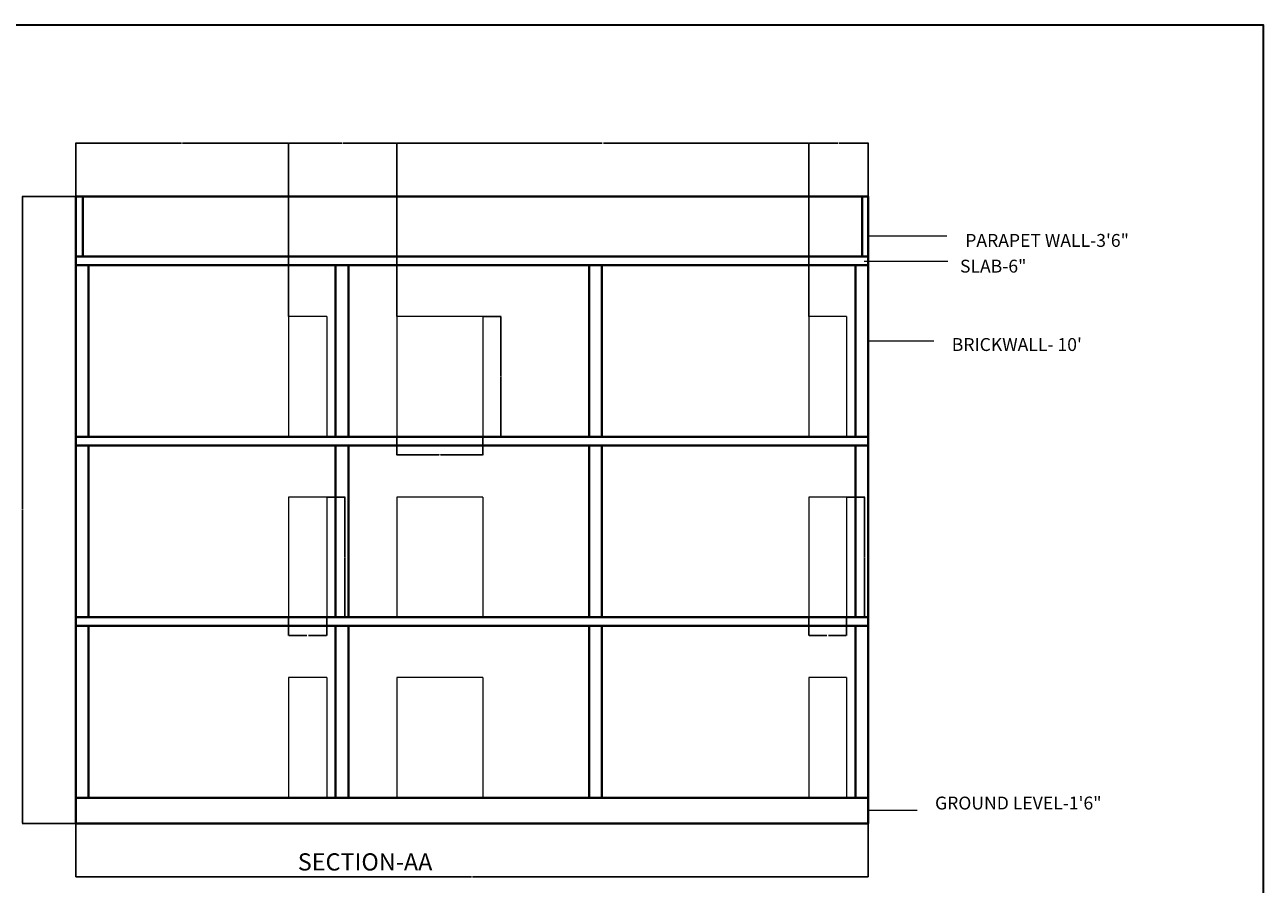
# Model space of a CAD drawing. Units: inches. Extents: x 2014 to 3678, y 870 to 2323.
# Tile 7 of 7: x 2813 to 3678, y 1723 to 2323. Entities that reach past the tile are written whole.
import ezdxf

# ---------------------------------------------------------------- set-up
doc = ezdxf.new("R2010")
doc.units = ezdxf.units.IN
for name, color, linetype, lineweight in [('A-ANNO-DIMS', 2, 'Continuous', 18), ('A-ANNO-SYMB', 2, 'Continuous', 18), ('A-ANNO-TEXT', 7, 'Continuous', 18), ('A-ANNO-TTLB', 7, 'Continuous', 35), ('A-SECT', 7, 'Continuous', 40), ('A-SECT-OPEN', 4, 'Continuous', 18)]:
    doc.layers.add(name, color=color, linetype=linetype, lineweight=lineweight)
doc.styles.get("Standard").update_dxf_attribs({"font": 'arial.ttf'})
doc.dimstyles.get("Standard").update_dxf_attribs({"dimtxt": 0.18, "dimasz": 0.18, "dimexe": 0.18, "dimexo": 0.0625, "dimgap": 0.09, "dimtad": 0, "dimtih": 1, "dimtoh": 1, "dimdec": 4, "dimzin": 0, "dimdsep": 46, "dimtxsty": 'Standard', "dimcen": 0.09, "dimadec": 0, "dimazin": 0, "dimtfac": 1, "dimtdec": 4, "dimtofl": 0, "dimtmove": 0, "dimatfit": 3, "dimfxl": 1, "dimtolj": 1, "dimtzin": 0, "dimarcsym": 0})

# ---------------------------------------------------------------- blocks, each defined once
blk = doc.blocks.new('SECT-OPENING-LAV-EAST')
for p, q in [((0, 84), (0, 0)), ((26.34, 84), (0, 84)), ((26.34, 84), (26.34, 0))]:
    blk.add_line(p, q)
blk = doc.blocks.new('SECT-OPENING-LAV-WEST')
for p, q in [((0, 84), (0, 0)), ((26.83, 84), (0, 84)), ((26.83, 84), (26.83, 0))]:
    blk.add_line(p, q)
blk = doc.blocks.new('SECT-OPENING-BED')
for p, q in [((0, 84), (0, 0)), ((60, 84), (0, 84)), ((60, 84), (60, 0))]:
    blk.add_line(p, q)
blk = doc.blocks.new('*D80')
at = {"layer": 'A-ANNO-DIMS', "color": 0, "lineweight": -2, "transparency": 16777216}
for p, q in [((3387.07, 1993.52), (3399.78, 1993.52)), ((3399.6, 1993.34), (3399.6, 1951.71)), ((3399.6, 1909.7), (3399.6, 1951.34)), ((3387.07, 1909.52), (3399.78, 1909.52))]:
    blk.add_line(p, q, dxfattribs=at)
at = {"layer": 'A-ANNO-DIMS', "color": 0, "transparency": 16777216}
for points in [[(3399.57, 1993.34), (3399.63, 1993.34), (3399.6, 1993.52)], [(3399.57, 1909.7), (3399.63, 1909.7), (3399.6, 1909.52)]]:
    blk.add_solid(points, dxfattribs=at)
at = {"layer": 'Defpoints', "color": 0, "transparency": 16777216}
for p in [(3387, 1993.52), (3399.6, 1993.52), (3387, 1909.52)]:
    blk.add_point(p, dxfattribs=at)
at = {"layer": 'A-ANNO-DIMS', "color": 0, "transparency": 16777216, "insert": (3399.6, 1951.52), "char_height": 0.18, "attachment_point": 5}
blk.add_mtext('\\A1;OPENING 84 TYP.', dxfattribs=at)
blk = doc.blocks.new('*D81')
at = {"layer": 'A-ANNO-DIMS', "color": 0, "lineweight": -2, "transparency": 16777216}
for p, q in [((3360.66, 1909.46), (3360.66, 1896.74)), ((3387, 1909.46), (3387, 1896.74)), ((3360.84, 1896.92), (3373.31, 1896.92)), ((3386.82, 1896.92), (3374.36, 1896.92))]:
    blk.add_line(p, q, dxfattribs=at)
at = {"layer": 'A-ANNO-DIMS', "color": 0, "transparency": 16777216}
for points in [[(3360.84, 1896.95), (3360.84, 1896.89), (3360.66, 1896.92)], [(3386.82, 1896.95), (3386.82, 1896.89), (3387, 1896.92)]]:
    blk.add_solid(points, dxfattribs=at)
at = {"layer": 'Defpoints', "color": 0, "transparency": 16777216}
for p in [(3360.66, 1909.52), (3387, 1909.52), (3387, 1896.92)]:
    blk.add_point(p, dxfattribs=at)
at = {"layer": 'A-ANNO-DIMS', "color": 0, "transparency": 16777216, "insert": (3373.83, 1896.92), "char_height": 0.18, "attachment_point": 5}
blk.add_mtext('\\A1;26 TYP.', dxfattribs=at)
blk = doc.blocks.new('*D82')
at = {"layer": 'A-ANNO-DIMS', "color": 0, "lineweight": -2, "transparency": 16777216}
for p, q in [((3024.17, 1993.52), (3036.89, 1993.52)), ((3036.71, 1993.34), (3036.71, 1951.71)), ((3036.71, 1909.7), (3036.71, 1951.34)), ((3024.17, 1909.52), (3036.89, 1909.52))]:
    blk.add_line(p, q, dxfattribs=at)
at = {"layer": 'A-ANNO-DIMS', "color": 0, "transparency": 16777216}
for points in [[(3036.68, 1993.34), (3036.74, 1993.34), (3036.71, 1993.52)], [(3036.68, 1909.7), (3036.74, 1909.7), (3036.71, 1909.52)]]:
    blk.add_solid(points, dxfattribs=at)
at = {"layer": 'Defpoints', "color": 0, "transparency": 16777216}
for p in [(3024.11, 1993.52), (3036.71, 1993.52), (3024.11, 1909.52)]:
    blk.add_point(p, dxfattribs=at)
at = {"layer": 'A-ANNO-DIMS', "color": 0, "transparency": 16777216, "insert": (3036.71, 1951.52), "char_height": 0.18, "attachment_point": 5}
blk.add_mtext('\\A1;OPENING 84 TYP.', dxfattribs=at)
blk = doc.blocks.new('*D83')
at = {"layer": 'A-ANNO-DIMS', "color": 0, "lineweight": -2, "transparency": 16777216}
for p, q in [((2997.28, 1909.46), (2997.28, 1896.74)), ((3024.11, 1909.46), (3024.11, 1896.74)), ((2997.46, 1896.92), (3010.16, 1896.92)), ((3023.93, 1896.92), (3011.22, 1896.92))]:
    blk.add_line(p, q, dxfattribs=at)
at = {"layer": 'A-ANNO-DIMS', "color": 0, "transparency": 16777216}
for points in [[(2997.46, 1896.95), (2997.46, 1896.89), (2997.28, 1896.92)], [(3023.93, 1896.95), (3023.93, 1896.89), (3024.11, 1896.92)]]:
    blk.add_solid(points, dxfattribs=at)
at = {"layer": 'Defpoints', "color": 0, "transparency": 16777216}
for p in [(2997.28, 1909.52), (3024.11, 1909.52), (3024.11, 1896.92)]:
    blk.add_point(p, dxfattribs=at)
at = {"layer": 'A-ANNO-DIMS', "color": 0, "transparency": 16777216, "insert": (3010.69, 1896.92), "char_height": 0.18, "attachment_point": 5}
blk.add_mtext('\\A1;27 TYP.', dxfattribs=at)
blk = doc.blocks.new('*D84')
at = {"layer": 'A-ANNO-DIMS', "color": 0, "lineweight": -2, "transparency": 16777216}
for p, q in [((3132.99, 2119.52), (3145.71, 2119.52)), ((3145.53, 2119.34), (3145.53, 2077.71)), ((3145.53, 2035.7), (3145.53, 2077.34)), ((3132.99, 2035.52), (3145.71, 2035.52))]:
    blk.add_line(p, q, dxfattribs=at)
at = {"layer": 'A-ANNO-DIMS', "color": 0, "transparency": 16777216}
for points in [[(3145.5, 2119.34), (3145.56, 2119.34), (3145.53, 2119.52)], [(3145.5, 2035.7), (3145.56, 2035.7), (3145.53, 2035.52)]]:
    blk.add_solid(points, dxfattribs=at)
at = {"layer": 'Defpoints', "color": 0, "transparency": 16777216}
for p in [(3132.93, 2119.52), (3145.53, 2119.52), (3132.93, 2035.52)]:
    blk.add_point(p, dxfattribs=at)
at = {"layer": 'A-ANNO-DIMS', "color": 0, "transparency": 16777216, "insert": (3145.53, 2077.52), "char_height": 0.18, "attachment_point": 5}
blk.add_mtext('\\A1;OPENING 84 TYP.', dxfattribs=at)
blk = doc.blocks.new('*D85')
at = {"layer": 'A-ANNO-DIMS', "color": 0, "lineweight": -2, "transparency": 16777216}
for p, q in [((3072.93, 2035.46), (3072.93, 2022.74)), ((3132.93, 2035.46), (3132.93, 2022.74)), ((3073.11, 2022.92), (3102.4, 2022.92)), ((3132.75, 2022.92), (3103.45, 2022.92))]:
    blk.add_line(p, q, dxfattribs=at)
at = {"layer": 'A-ANNO-DIMS', "color": 0, "transparency": 16777216}
for points in [[(3073.11, 2022.95), (3073.11, 2022.89), (3072.93, 2022.92)], [(3132.75, 2022.95), (3132.75, 2022.89), (3132.93, 2022.92)]]:
    blk.add_solid(points, dxfattribs=at)
at = {"layer": 'Defpoints', "color": 0, "transparency": 16777216}
for p in [(3072.93, 2035.52), (3132.93, 2035.52), (3132.93, 2022.92)]:
    blk.add_point(p, dxfattribs=at)
at = {"layer": 'A-ANNO-DIMS', "color": 0, "transparency": 16777216, "insert": (3102.93, 2022.92), "char_height": 0.18, "attachment_point": 5}
blk.add_mtext('\\A1;60 TYP.', dxfattribs=at)
blk = doc.blocks.new('*D114')
at = {"layer": 'A-ANNO-DIMS', "color": 0, "lineweight": -2, "transparency": 16777216}
for p, q in [((2848.67, 1765.46), (2848.67, 1728.19)), ((3402.17, 1765.46), (3402.17, 1728.19)), ((2848.85, 1728.37), (3125.03, 1728.37)), ((3401.99, 1728.37), (3125.82, 1728.37))]:
    blk.add_line(p, q, dxfattribs=at)
at = {"layer": 'A-ANNO-DIMS', "color": 0, "transparency": 16777216}
for points in [[(2848.85, 1728.4), (2848.85, 1728.34), (2848.67, 1728.37)], [(3401.99, 1728.4), (3401.99, 1728.34), (3402.17, 1728.37)]]:
    blk.add_solid(points, dxfattribs=at)
at = {"layer": 'Defpoints', "color": 0, "transparency": 16777216}
for p in [(2848.67, 1765.52), (3402.17, 1765.52), (3402.17, 1728.37)]:
    blk.add_point(p, dxfattribs=at)
at = {"layer": 'A-ANNO-DIMS', "color": 0, "transparency": 16777216, "insert": (3125.42, 1728.37), "char_height": 0.18, "attachment_point": 5}
blk.add_mtext('\\A1;553.5', dxfattribs=at)
blk = doc.blocks.new('*D115')
at = {"layer": 'A-ANNO-DIMS', "color": 0, "lineweight": -2, "transparency": 16777216}
for p, q in [((2848.61, 2203.52), (2811.34, 2203.52)), ((2811.52, 2203.34), (2811.52, 1984.71)), ((2811.52, 1765.7), (2811.52, 1984.34)), ((2848.61, 1765.52), (2811.34, 1765.52))]:
    blk.add_line(p, q, dxfattribs=at)
at = {"layer": 'A-ANNO-DIMS', "color": 0, "transparency": 16777216}
for points in [[(2811.49, 2203.34), (2811.55, 2203.34), (2811.52, 2203.52)], [(2811.49, 1765.7), (2811.55, 1765.7), (2811.52, 1765.52)]]:
    blk.add_solid(points, dxfattribs=at)
at = {"layer": 'Defpoints', "color": 0, "transparency": 16777216}
for p in [(2811.52, 2203.52), (2848.67, 2203.52), (2848.67, 1765.52)]:
    blk.add_point(p, dxfattribs=at)
at = {"layer": 'A-ANNO-DIMS', "color": 0, "transparency": 16777216, "insert": (2811.52, 1984.52), "char_height": 0.18, "attachment_point": 5}
blk.add_mtext('\\A1;438', dxfattribs=at)
blk = doc.blocks.new('*D116')
at = {"layer": 'A-ANNO-DIMS', "color": 0, "lineweight": -2, "transparency": 16777216}
for p, q in [((2848.67, 2203.59), (2848.67, 2240.85)), ((2848.85, 2240.67), (2922.59, 2240.67)), ((2997.1, 2240.67), (2923.36, 2240.67)), ((2997.28, 2119.59), (2997.28, 2240.85))]:
    blk.add_line(p, q, dxfattribs=at)
at = {"layer": 'A-ANNO-DIMS', "color": 0, "transparency": 16777216}
for points in [[(2848.85, 2240.7), (2848.85, 2240.64), (2848.67, 2240.67)], [(2997.1, 2240.7), (2997.1, 2240.64), (2997.28, 2240.67)]]:
    blk.add_solid(points, dxfattribs=at)
at = {"layer": 'Defpoints', "color": 0, "transparency": 16777216}
for p in [(2997.28, 2240.67), (2848.67, 2203.52), (2997.28, 2119.52)]:
    blk.add_point(p, dxfattribs=at)
at = {"layer": 'A-ANNO-DIMS', "color": 0, "transparency": 16777216, "insert": (2922.97, 2240.67), "char_height": 0.18, "attachment_point": 5}
blk.add_mtext('\\A1;148.6', dxfattribs=at)
blk = doc.blocks.new('*D117')
at = {"layer": 'A-ANNO-DIMS', "color": 0, "lineweight": -2, "transparency": 16777216}
for p, q in [((2997.28, 2119.59), (2997.28, 2240.85)), ((2997.46, 2240.67), (3034.71, 2240.67)), ((3072.75, 2240.67), (3035.49, 2240.67)), ((3072.93, 2119.59), (3072.93, 2240.85))]:
    blk.add_line(p, q, dxfattribs=at)
at = {"layer": 'A-ANNO-DIMS', "color": 0, "transparency": 16777216}
for points in [[(2997.46, 2240.7), (2997.46, 2240.64), (2997.28, 2240.67)], [(3072.75, 2240.7), (3072.75, 2240.64), (3072.93, 2240.67)]]:
    blk.add_solid(points, dxfattribs=at)
at = {"layer": 'Defpoints', "color": 0, "transparency": 16777216}
for p in [(3072.93, 2240.67), (2997.28, 2119.52), (3072.93, 2119.52)]:
    blk.add_point(p, dxfattribs=at)
at = {"layer": 'A-ANNO-DIMS', "color": 0, "transparency": 16777216, "insert": (3035.1, 2240.67), "char_height": 0.18, "attachment_point": 5}
blk.add_mtext('\\A1;75.65', dxfattribs=at)
blk = doc.blocks.new('*D118')
at = {"layer": 'A-ANNO-DIMS', "color": 0, "lineweight": -2, "transparency": 16777216}
for p, q in [((3072.93, 2119.59), (3072.93, 2240.85)), ((3073.11, 2240.67), (3216.33, 2240.67)), ((3360.48, 2240.67), (3217.26, 2240.67)), ((3360.66, 2119.59), (3360.66, 2240.85))]:
    blk.add_line(p, q, dxfattribs=at)
at = {"layer": 'A-ANNO-DIMS', "color": 0, "transparency": 16777216}
for points in [[(3073.11, 2240.7), (3073.11, 2240.64), (3072.93, 2240.67)], [(3360.48, 2240.7), (3360.48, 2240.64), (3360.66, 2240.67)]]:
    blk.add_solid(points, dxfattribs=at)
at = {"layer": 'Defpoints', "color": 0, "transparency": 16777216}
for p in [(3360.66, 2240.67), (3072.93, 2119.52), (3360.66, 2119.52)]:
    blk.add_point(p, dxfattribs=at)
at = {"layer": 'A-ANNO-DIMS', "color": 0, "transparency": 16777216, "insert": (3216.8, 2240.67), "char_height": 0.18, "attachment_point": 5}
blk.add_mtext('\\A1;287.74', dxfattribs=at)
blk = doc.blocks.new('*D119')
at = {"layer": 'A-ANNO-DIMS', "color": 0, "lineweight": -2, "transparency": 16777216}
for p, q in [((3360.66, 2119.59), (3360.66, 2240.85)), ((3360.84, 2240.67), (3381.04, 2240.67)), ((3401.99, 2240.67), (3381.8, 2240.67)), ((3402.17, 2203.59), (3402.17, 2240.85))]:
    blk.add_line(p, q, dxfattribs=at)
at = {"layer": 'A-ANNO-DIMS', "color": 0, "transparency": 16777216}
for points in [[(3360.84, 2240.7), (3360.84, 2240.64), (3360.66, 2240.67)], [(3401.99, 2240.7), (3401.99, 2240.64), (3402.17, 2240.67)]]:
    blk.add_solid(points, dxfattribs=at)
at = {"layer": 'Defpoints', "color": 0, "transparency": 16777216}
for p in [(3402.17, 2240.67), (3402.17, 2203.52), (3360.66, 2119.52)]:
    blk.add_point(p, dxfattribs=at)
at = {"layer": 'A-ANNO-DIMS', "color": 0, "transparency": 16777216, "insert": (3381.42, 2240.67), "char_height": 0.18, "attachment_point": 5}
blk.add_mtext('\\A1;41.51', dxfattribs=at)

msp = doc.modelspace()

# ---------------------------------------------------------------- linework, layer by layer
at = {"layer": 'A-ANNO-SYMB'}
for p, q in [((3402.1718, 2175.8362), (3456.966, 2175.8362)), ((3399.338, 2158.1977), (3457.7977, 2158.1977)), ((3402.1718, 2102.5752), (3448.0271, 2102.5752)), ((3402.1718, 1774.9062), (3436.4174, 1774.9062))]:
    msp.add_line(p, q, dxfattribs=at)
at = {"layer": 'A-ANNO-TTLB'}
msp.add_lwpolyline([(2014.0556, 2323.3638), (3678.0069, 2323.3638), (3678.0069, 869.855), (2014.0556, 869.855)], close=True, dxfattribs=at)
at = {"layer": 'A-SECT'}
for p, q in [((2848.6718, 2203.5235), (2848.6718, 2017.5235)), ((3402.1718, 2203.5235), (2848.6718, 2203.5235)), ((2853.6051, 2161.5235), (2853.6051, 2203.5235)), ((3397.8601, 2161.5235), (3397.8601, 2203.5235)), ((3402.1718, 2203.5235), (3402.1718, 2017.5235)), ((3402.1718, 2161.5235), (2848.6718, 2161.5235)), ((3402.1718, 2155.5235), (2848.6718, 2155.5235)), ((2857.6718, 2155.5235), (2857.6718, 2035.5235)), ((3030.1718, 2155.5235), (3030.1718, 2035.5235)), ((3039.1718, 2155.5235), (3039.1718, 2035.5235)), ((3207.1718, 2155.5235), (3207.1718, 2035.5235)), ((3216.1718, 2155.5235), (3216.1718, 2035.5235)), ((3393.1718, 2155.5235), (3393.1718, 2035.5235)), ((2848.6718, 2077.5235), (2848.6718, 1891.5235)), ((3402.1718, 2077.5235), (3402.1718, 1891.5235)), ((3402.1718, 2035.5235), (2848.6718, 2035.5235)), ((3402.1718, 2029.5235), (2848.6718, 2029.5235)), ((2857.6718, 2029.5235), (2857.6718, 1909.5235)), ((3030.1718, 2029.5235), (3030.1718, 1909.5235)), ((3039.1718, 2029.5235), (3039.1718, 1909.5235)), ((3207.1718, 2029.5235), (3207.1718, 1909.5235)), ((3216.1718, 2029.5235), (3216.1718, 1909.5235)), ((3393.1718, 2029.5235), (3393.1718, 1909.5235)), ((2848.6718, 1951.5235), (2848.6718, 1765.5235)), ((3402.1718, 1951.5235), (3402.1718, 1765.5235)), ((3402.1718, 1909.5235), (2848.6718, 1909.5235)), ((3402.1718, 1903.5235), (2848.6718, 1903.5235)), ((2857.6718, 1903.5235), (2857.6718, 1783.5235)), ((3030.1718, 1903.5235), (3030.1718, 1783.5235)), ((3039.1718, 1903.5235), (3039.1718, 1783.5235)), ((3207.1718, 1903.5235), (3207.1718, 1783.5235)), ((3216.1718, 1903.5235), (3216.1718, 1783.5235)), ((3393.1718, 1903.5235), (3393.1718, 1783.5235)), ((3402.1718, 1783.5235), (2848.6718, 1783.5235)), ((3402.1718, 1765.5235), (2848.6718, 1765.5235))]:
    msp.add_line(p, q, dxfattribs=at)

# ---------------------------------------------------------------- block references
at = {"layer": 'A-SECT-OPEN'}
for name, p in [('SECT-OPENING-LAV-WEST', (2997.276, 2035.523)), ('SECT-OPENING-BED', (3072.926, 2035.523)), ('SECT-OPENING-LAV-EAST', (3360.665, 2035.523)), ('SECT-OPENING-LAV-WEST', (2997.276, 1909.523)), ('SECT-OPENING-BED', (3072.926, 1909.523)), ('SECT-OPENING-LAV-EAST', (3360.665, 1909.523)), ('SECT-OPENING-LAV-WEST', (2997.276, 1783.523)), ('SECT-OPENING-BED', (3072.926, 1783.523)), ('SECT-OPENING-LAV-EAST', (3360.665, 1783.523))]:
    msp.add_blockref(name, p, dxfattribs=at)

# ---------------------------------------------------------------- texts
at = {"layer": 'A-ANNO-TEXT', "attachment_point": 1}
for s, width, insert, char_height in [('PARAPET WALL-3\'6"', 403.726463, (3469.9111, 2177.2392), 9), ('SLAB-6"', 43.616049, (3466.2258, 2159.2828), 9), ("BRICKWALL- 10'", 128.818942, (3460.4898, 2104.5416), 9), ('GROUND LEVEL-1\'6"', 156.075409, (3448.8136, 1784.2972), 9), ('SECTION-AA', 322.035475, (3003.7521, 1744.687), 12)]:
    msp.add_mtext_dynamic_manual_height_columns(s, width=width, gutter_width=12.5, heights=[0], dxfattribs=dict(at, insert=insert, char_height=char_height))

# ---------------------------------------------------------------- dimensions: what is measured, and where the dimension line sits
at = {"layer": 'A-ANNO-DIMS'}
for base, p1, p2, override, picture, middle in [((2997.2758, 2240.6735), (2848.6718, 2203.5235), (2997.2758, 2119.5235), {"dimdec": 1, "dimlfac": 1, "dimrnd": 0, "dimzin": 0, "dimdsep": 46, "dimlunit": 2}, '*D116', (2922.9738, 2240.6735)), ((3072.9257, 2240.6735), (2997.2758, 2119.5235), (3072.9257, 2119.5235), {"dimdec": 2, "dimlfac": 1, "dimrnd": 0, "dimzin": 0, "dimdsep": 46, "dimlunit": 2}, '*D117', (3035.1008, 2240.6735)), ((3360.6647, 2240.6735), (3072.9257, 2119.5235), (3360.6647, 2119.5235), {"dimdec": 2, "dimlfac": 1, "dimrnd": 0, "dimzin": 0, "dimdsep": 46, "dimlunit": 2}, '*D118', (3216.7952, 2240.6735)), ((3402.1718, 2240.6735), (3360.6647, 2119.5235), (3402.1718, 2203.5235), {"dimdec": 2, "dimlfac": 1, "dimrnd": 0, "dimzin": 0, "dimdsep": 46, "dimlunit": 2}, '*D119', (3381.4182, 2240.6735)), ((3402.1718, 1728.3735), (2848.6718, 1765.5235), (3402.1718, 1765.5235), {"dimdec": 1, "dimlfac": 1, "dimrnd": 0, "dimzin": 0, "dimdsep": 46, "dimlunit": 2}, '*D114', (3125.4218, 1728.3735))]:
    dim = msp.add_linear_dim(base=base, p1=p1, p2=p2, dimstyle='Standard', override=override, dxfattribs=at)
    dim.commit()
    dim.dimension.update_dxf_attribs({"geometry": picture, "text_midpoint": middle})
dim = msp.add_linear_dim(base=(2811.5218, 2203.5235), p1=(2848.6718, 1765.5235), p2=(2848.6718, 2203.5235), angle=90, dimstyle='Standard', override={"dimdec": 0, "dimlfac": 1, "dimrnd": 0, "dimzin": 0, "dimdsep": 46, "dimlunit": 2}, dxfattribs=at)
dim.commit()
dim.dimension.update_dxf_attribs({"geometry": '*D115', "text_midpoint": (2811.5218, 1984.5235)})
for base, p1, p2, picture, middle in [((3145.5257, 2119.5235), (3132.9257, 2035.5235), (3132.9257, 2119.5235), '*D84', (3145.5257, 2077.5235)), ((3036.7088, 1993.5235), (3024.1088, 1909.5235), (3024.1088, 1993.5235), '*D82', (3036.7088, 1951.5235)), ((3399.6048, 1993.5235), (3387.0048, 1909.5235), (3387.0048, 1993.5235), '*D80', (3399.6048, 1951.5235))]:
    dim = msp.add_linear_dim(base=base, p1=p1, p2=p2, angle=90, text='OPENING <> TYP.', dimstyle='Standard', override={"dimdec": 0, "dimlfac": 1, "dimrnd": 0, "dimzin": 0, "dimdsep": 46, "dimlunit": 2}, dxfattribs=at)
    dim.commit()
    dim.dimension.update_dxf_attribs({"geometry": picture, "text_midpoint": middle})
for base, p1, p2, picture, middle in [((3132.9257, 2022.9235), (3072.9257, 2035.5235), (3132.9257, 2035.5235), '*D85', (3102.9257, 2022.9235)), ((3024.1088, 1896.9235), (2997.2758, 1909.5235), (3024.1088, 1909.5235), '*D83', (3010.6923, 1896.9235)), ((3387.0048, 1896.9235), (3360.6647, 1909.5235), (3387.0048, 1909.5235), '*D81', (3373.8348, 1896.9235))]:
    dim = msp.add_linear_dim(base=base, p1=p1, p2=p2, text='<> TYP.', dimstyle='Standard', override={"dimdec": 0, "dimlfac": 1, "dimrnd": 0, "dimzin": 0, "dimdsep": 46, "dimlunit": 2}, dxfattribs=at)
    dim.commit()
    dim.dimension.update_dxf_attribs({"geometry": picture, "text_midpoint": middle})

doc.saveas('drawing.dxf')
